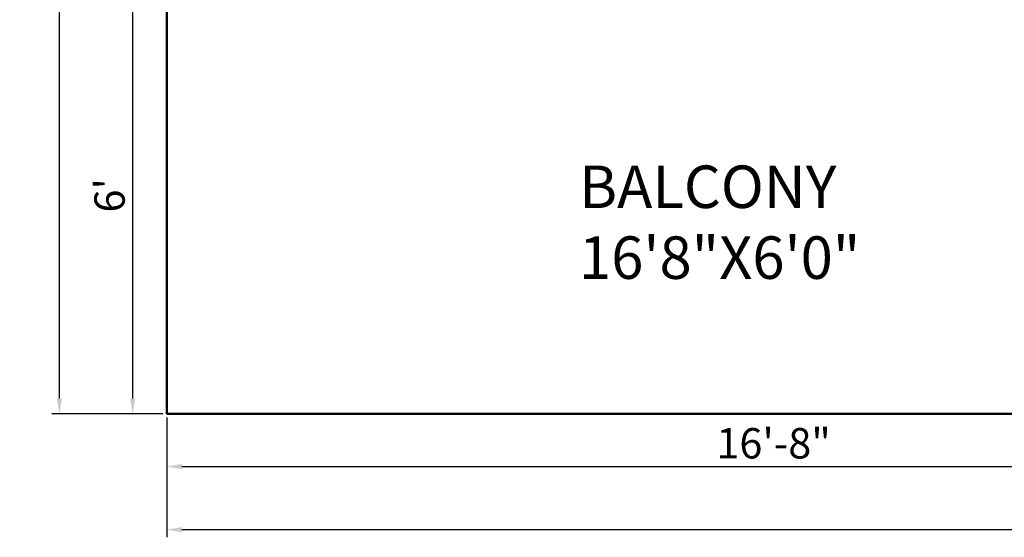
# Model space of a CAD drawing. Units: inches. Extents: x 3064 to 19385, y 846 to 15425.
# Tile 65 of 108: x 6445 to 6607, y 1476 to 1561. Entities that reach past the tile are written whole.
import ezdxf

# ---------------------------------------------------------------- set-up
doc = ezdxf.new("R2010")
doc.units = ezdxf.units.IN
for name, color, linetype, lineweight in [('A-ANNO-DIMS', 2, 'Continuous', 18), ('A-AREA-IDEN', 3, 'Continuous', 18), ('A-WALL', 7, 'Continuous', 50)]:
    doc.layers.add(name, color=color, linetype=linetype, lineweight=lineweight)
doc.styles.get("Standard").update_dxf_attribs({"font": 'arial.ttf'})
doc.dimstyles.new('ISO-25', dxfattribs={"dimtxt": 9, "dimasz": 2.5, "dimexe": 1.25, "dimexo": 0.625, "dimtad": 1, "dimdec": 1, "dimlunit": 3, "dimtxsty": 'Standard', "dimcen": 2.5, "dimadec": 0, "dimazin": 0, "dimtfac": 1, "dimtdec": 1, "dimtmove": 0, "dimatfit": 3, "dimfxl": 1, "dimarcsym": 0})

# ---------------------------------------------------------------- blocks, each defined once
blk = doc.blocks.new('*D379')
at = {"layer": 'A-ANNO-DIMS', "color": 0, "lineweight": -2, "transparency": 16777216}
for p, q in [((6468.41, 1567.99), (6462.18, 1567.99)), ((6463.43, 1498.49), (6463.43, 1565.49)), ((6468.41, 1495.99), (6462.18, 1495.99))]:
    blk.add_line(p, q, dxfattribs=at)
at = {"layer": 'A-ANNO-DIMS', "color": 0, "transparency": 16777216}
for points in [[(6463.02, 1565.49), (6463.85, 1565.49), (6463.43, 1567.99)], [(6463.02, 1498.49), (6463.85, 1498.49), (6463.43, 1495.99)]]:
    blk.add_solid(points, dxfattribs=at)
at = {"layer": 'Defpoints', "color": 0, "transparency": 16777216}
for p in [(6463.43, 1567.99), (6469.03, 1567.99), (6469.03, 1495.99)]:
    blk.add_point(p, dxfattribs=at)
at = {"layer": 'A-ANNO-DIMS', "color": 0, "transparency": 16777216, "insert": (6460.26, 1531.99), "char_height": 5, "attachment_point": 5, "rotation": 90}
blk.add_mtext("6'", dxfattribs=at)
blk = doc.blocks.new('*D370')
at = {"layer": 'A-ANNO-DIMS', "color": 0, "lineweight": -2, "transparency": 16777216}
for p, q in [((6468.41, 1987.99), (6450.1, 1987.99)), ((6451.35, 1498.49), (6451.35, 1985.49)), ((6468.41, 1495.99), (6450.1, 1495.99))]:
    blk.add_line(p, q, dxfattribs=at)
at = {"layer": 'A-ANNO-DIMS', "color": 0, "transparency": 16777216}
for points in [[(6450.94, 1985.49), (6451.77, 1985.49), (6451.35, 1987.99)], [(6450.94, 1498.49), (6451.77, 1498.49), (6451.35, 1495.99)]]:
    blk.add_solid(points, dxfattribs=at)
at = {"layer": 'Defpoints', "color": 0, "transparency": 16777216}
for p in [(6451.35, 1987.99), (6469.03, 1987.99), (6469.03, 1495.99)]:
    blk.add_point(p, dxfattribs=at)
at = {"layer": 'A-ANNO-DIMS', "color": 0, "transparency": 16777216, "insert": (6448.22, 1741.99), "char_height": 5, "attachment_point": 5, "rotation": 90}
blk.add_mtext("41'", dxfattribs=at)
blk = doc.blocks.new('*D359')
at = {"layer": 'A-ANNO-DIMS', "color": 0, "lineweight": -2, "transparency": 16777216}
for p, q in [((6469.03, 1495.36), (6469.03, 1486.07)), ((6669.03, 1495.36), (6669.03, 1486.07)), ((6471.53, 1487.32), (6666.53, 1487.32))]:
    blk.add_line(p, q, dxfattribs=at)
at = {"layer": 'A-ANNO-DIMS', "color": 0, "transparency": 16777216}
for points in [[(6471.53, 1487.73), (6471.53, 1486.9), (6469.03, 1487.32)], [(6666.53, 1487.73), (6666.53, 1486.9), (6669.03, 1487.32)]]:
    blk.add_solid(points, dxfattribs=at)
at = {"layer": 'Defpoints', "color": 0, "transparency": 16777216}
for p in [(6469.03, 1495.99), (6669.03, 1495.99), (6669.03, 1487.32)]:
    blk.add_point(p, dxfattribs=at)
at = {"layer": 'A-ANNO-DIMS', "color": 0, "transparency": 16777216, "insert": (6569.03, 1490.49), "char_height": 5, "attachment_point": 5}
blk.add_mtext('16\'-8"', dxfattribs=at)
blk = doc.blocks.new('*D342')
at = {"layer": 'A-ANNO-DIMS', "color": 0, "lineweight": -2, "transparency": 16777216}
for p, q in [((6469.03, 1495.36), (6469.03, 1475.66)), ((6811.03, 1495.36), (6811.03, 1475.66)), ((6808.53, 1476.91), (6471.53, 1476.91))]:
    blk.add_line(p, q, dxfattribs=at)
at = {"layer": 'A-ANNO-DIMS', "color": 0, "transparency": 16777216}
for points in [[(6471.53, 1477.32), (6471.53, 1476.49), (6469.03, 1476.91)], [(6808.53, 1477.32), (6808.53, 1476.49), (6811.03, 1476.91)]]:
    blk.add_solid(points, dxfattribs=at)
at = {"layer": 'Defpoints', "color": 0, "transparency": 16777216}
for p in [(6469.03, 1495.99), (6811.03, 1495.99), (6469.03, 1476.91)]:
    blk.add_point(p, dxfattribs=at)
at = {"layer": 'A-ANNO-DIMS', "color": 0, "transparency": 16777216, "insert": (6640.03, 1480.08), "char_height": 5, "attachment_point": 5}
blk.add_mtext('28\'-6"', dxfattribs=at)

msp = doc.modelspace()

# ---------------------------------------------------------------- linework, layer by layer
at = {"layer": 'A-WALL'}
for p, q in [((6469.03, 1567.99), (6469.03, 1495.99)), ((6469.03, 1495.99), (6811.03, 1495.99))]:
    msp.add_line(p, q, dxfattribs=at)

# ---------------------------------------------------------------- texts
at = {"layer": 'A-AREA-IDEN', "insert": (6536.97, 1536.89), "char_height": 7, "attachment_point": 1}
msp.add_mtext_dynamic_manual_height_columns('BALCONY\\P16\'8"X6\'0"', width=67.5924, gutter_width=12.5, heights=[0], dxfattribs=at)

# ---------------------------------------------------------------- dimensions: what is measured, and where the dimension line sits
at = {"layer": 'A-ANNO-DIMS'}
for base, p2, picture, middle in [((6451.35, 1987.99), (6469.03, 1987.99), '*D370', (6448.22, 1741.99)), ((6463.43, 1567.99), (6469.03, 1567.99), '*D379', (6460.26, 1531.99))]:
    dim = msp.add_linear_dim(base=base, p1=(6469.03, 1495.99), p2=p2, angle=90, dimstyle='ISO-25', override={"dimtxt": 5, "dimclrd": 0, "dimclre": 0, "dimclrt": 0}, dxfattribs=at)
    dim.commit()
    dim.dimension.update_dxf_attribs({"geometry": picture, "text_midpoint": middle})
for base, p1, p2, picture, middle in [((6669.03, 1487.32), (6469.03, 1495.99), (6669.03, 1495.99), '*D359', (6569.03, 1490.49)), ((6469.03, 1476.91), (6811.03, 1495.99), (6469.03, 1495.99), '*D342', (6640.03, 1480.08))]:
    dim = msp.add_linear_dim(base=base, p1=p1, p2=p2, dimstyle='ISO-25', override={"dimtxt": 5, "dimclrd": 0, "dimclre": 0, "dimclrt": 0}, dxfattribs=at)
    dim.commit()
    dim.dimension.update_dxf_attribs({"geometry": picture, "text_midpoint": middle})

doc.saveas('drawing.dxf')
